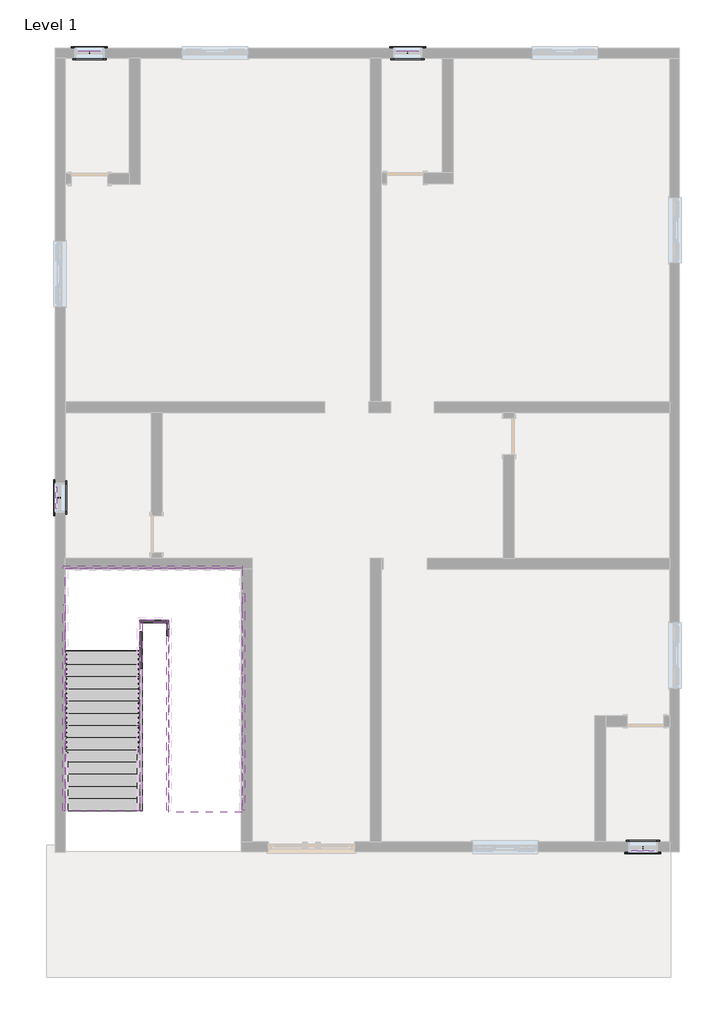
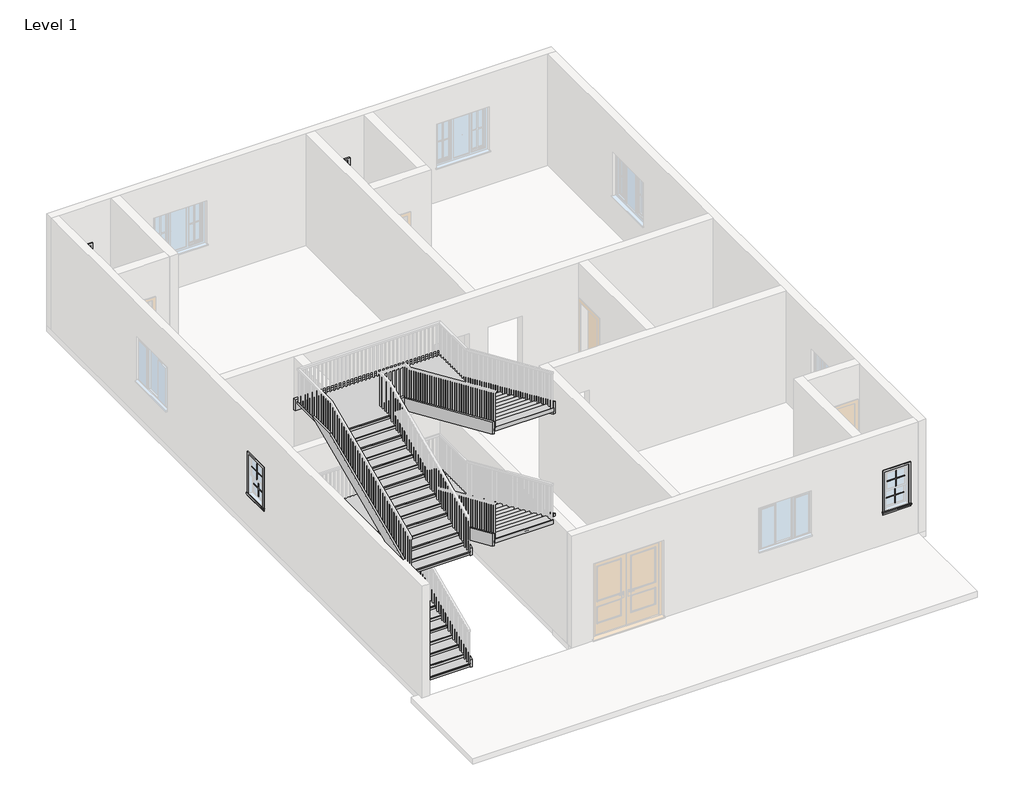
# One storey, part 6 of 6: 16 proxies, 12 members, 2 stair flights.
"""IFC4 building model written with IfcOpenShell, lengths in millimetres."""

from ifc_helpers import new_model, si_unit, frame, origin, place, context, project, spatial, polyline, outline, extrude, transform, mapped, element, save
from components import muntin_pattern_2x2_muntin_pattern_2x2_eba6c5fb, trim_window_exterior_flat_with_sill_278e6a94, trim_window_interior_flat_picture_frame_e9fd5f45, stair_flight_b71c2a3e, stair_flight_f7f46773

model = new_model("IFC4")

# Units and contexts
model_context = context("Model", 3, world=origin())
ifc_project = project(units=[si_unit("LENGTHUNIT", "METRE", prefix="MILLI")], contexts=[model_context])

# Site, building, storey
site = spatial("IfcSite", under=ifc_project)
building = spatial("IfcBuilding", under=site)
storey = spatial("IfcBuildingStorey", under=building, Name="Level 1", Elevation=0.0)

# Proxies
placement = place(None, origin())
muntin_pattern_2x2_muntin_pattern_2x2_shape = muntin_pattern_2x2_muntin_pattern_2x2_eba6c5fb(model_context)
element("IfcBuildingElementProxy", 1, Name="Muntin Pattern_2x2 : Muntin Pattern_2x2", ObjectType="Muntin Pattern_2x2 : Muntin Pattern_2x2", at=placement, inside=storey, context=model_context, shape_type="MappedRepresentation", body=[
    mapped(muntin_pattern_2x2_muntin_pattern_2x2_shape, transform((-7722.7165084, -455.2217109, 1470.025), x_axis=(0.0, 1.0, 0.0), y_axis=(-1.0, 0.0, 0.0), z_axis=(0.0, 0.0, 1.0))),
])
element("IfcBuildingElementProxy", 2, Name="Muntin Pattern_2x2 : Muntin Pattern_2x2", ObjectType="Muntin Pattern_2x2 : Muntin Pattern_2x2", at=placement, inside=storey, context=model_context, shape_type="MappedRepresentation", body=[
    mapped(muntin_pattern_2x2_muntin_pattern_2x2_shape, transform((-7678.2665084, -455.2217109, 990.6), x_axis=(0.0, 1.0, 0.0), y_axis=(-1.0, 0.0, 0.0), z_axis=(0.0, 0.0, 1.0))),
])
element("IfcBuildingElementProxy", 3, Name="Muntin Pattern_2x2 : Muntin Pattern_2x2", ObjectType="Muntin Pattern_2x2 : Muntin Pattern_2x2", at=placement, inside=storey, context=model_context, shape_type="MappedRepresentation", body=[
    mapped(muntin_pattern_2x2_muntin_pattern_2x2_shape, transform((-7046.4415084, 8872.5685985, 1470.025), x_axis=(1.0, 0.0, 0.0), y_axis=(0.0, 1.0, 0.0), z_axis=(0.0, 0.0, 1.0))),
])
element("IfcBuildingElementProxy", 4, Name="Muntin Pattern_2x2 : Muntin Pattern_2x2", ObjectType="Muntin Pattern_2x2 : Muntin Pattern_2x2", at=placement, inside=storey, context=model_context, shape_type="MappedRepresentation", body=[
    mapped(muntin_pattern_2x2_muntin_pattern_2x2_shape, transform((-7046.4415084, 8828.1185985, 990.6), x_axis=(1.0, 0.0, 0.0), y_axis=(0.0, 1.0, 0.0), z_axis=(0.0, 0.0, 1.0))),
])
element("IfcBuildingElementProxy", 5, Name="Muntin Pattern_2x2 : Muntin Pattern_2x2", ObjectType="Muntin Pattern_2x2 : Muntin Pattern_2x2", at=placement, inside=storey, context=model_context, shape_type="MappedRepresentation", body=[
    mapped(muntin_pattern_2x2_muntin_pattern_2x2_shape, transform((-417.0415084, 8872.5685985, 1470.025), x_axis=(1.0, 0.0, 0.0), y_axis=(0.0, 1.0, 0.0), z_axis=(0.0, 0.0, 1.0))),
])
element("IfcBuildingElementProxy", 6, Name="Muntin Pattern_2x2 : Muntin Pattern_2x2", ObjectType="Muntin Pattern_2x2 : Muntin Pattern_2x2", at=placement, inside=storey, context=model_context, shape_type="MappedRepresentation", body=[
    mapped(muntin_pattern_2x2_muntin_pattern_2x2_shape, transform((-417.0415084, 8828.1185985, 990.6), x_axis=(1.0, 0.0, 0.0), y_axis=(0.0, 1.0, 0.0), z_axis=(0.0, 0.0, 1.0))),
])
element("IfcBuildingElementProxy", 7, Name="Muntin Pattern_2x2 : Muntin Pattern_2x2", ObjectType="Muntin Pattern_2x2 : Muntin Pattern_2x2", at=placement, inside=storey, context=model_context, shape_type="MappedRepresentation", body=[
    mapped(muntin_pattern_2x2_muntin_pattern_2x2_shape, transform((4485.1584916, -7796.1814015, 1470.025), x_axis=(-1.0, 0.0, 0.0), y_axis=(0.0, -1.0, 0.0), z_axis=(0.0, 0.0, 1.0))),
])
element("IfcBuildingElementProxy", 8, Name="Muntin Pattern_2x2 : Muntin Pattern_2x2", ObjectType="Muntin Pattern_2x2 : Muntin Pattern_2x2", at=placement, inside=storey, context=model_context, shape_type="MappedRepresentation", body=[
    mapped(muntin_pattern_2x2_muntin_pattern_2x2_shape, transform((4485.1584916, -7751.7314015, 990.6), x_axis=(-1.0, 0.0, 0.0), y_axis=(0.0, -1.0, 0.0), z_axis=(0.0, 0.0, 1.0))),
])
trim_window_exterior_flat_with_sill_shape = trim_window_exterior_flat_with_sill_278e6a94(model_context)
element("IfcBuildingElementProxy", 9, Name="Trim-Window-Exterior-Flat : with Sill", ObjectType="Trim-Window-Exterior-Flat : with Sill", at=placement, inside=storey, context=model_context, shape_type="MappedRepresentation", body=[
    mapped(trim_window_exterior_flat_with_sill_shape, transform((-7757.6415084, -455.2217109, 1981.2), x_axis=(0.0, -1.0, 0.0), y_axis=(0.0, 0.0, 1.0), z_axis=(-1.0, 0.0, 0.0))),
])
element("IfcBuildingElementProxy", 10, Name="Trim-Window-Exterior-Flat : with Sill", ObjectType="Trim-Window-Exterior-Flat : with Sill", at=placement, inside=storey, context=model_context, shape_type="MappedRepresentation", body=[
    mapped(trim_window_exterior_flat_with_sill_shape, transform((-7046.4415084, 8907.4935985, 1981.2), x_axis=(-1.0, 0.0, 0.0), y_axis=(0.0, 0.0, 1.0), z_axis=(0.0, 1.0, 0.0))),
])
element("IfcBuildingElementProxy", 11, Name="Trim-Window-Exterior-Flat : with Sill", ObjectType="Trim-Window-Exterior-Flat : with Sill", at=placement, inside=storey, context=model_context, shape_type="MappedRepresentation", body=[
    mapped(trim_window_exterior_flat_with_sill_shape, transform((-417.0415084, 8907.4935985, 1981.2), x_axis=(-1.0, 0.0, 0.0), y_axis=(0.0, 0.0, 1.0), z_axis=(0.0, 1.0, 0.0))),
])
element("IfcBuildingElementProxy", 12, Name="Trim-Window-Exterior-Flat : with Sill", ObjectType="Trim-Window-Exterior-Flat : with Sill", at=placement, inside=storey, context=model_context, shape_type="MappedRepresentation", body=[
    mapped(trim_window_exterior_flat_with_sill_shape, transform((4485.1584916, -7831.1064015, 1981.2), x_axis=(1.0, 0.0, 0.0), y_axis=(0.0, 0.0, 1.0), z_axis=(0.0, -1.0, 0.0))),
])
trim_window_interior_flat_picture_frame_shape = trim_window_interior_flat_picture_frame_e9fd5f45(model_context)
element("IfcBuildingElementProxy", 13, Name="Trim-Window-Interior-Flat : Picture Frame", ObjectType="Trim-Window-Interior-Flat : Picture Frame", at=placement, inside=storey, context=model_context, shape_type="MappedRepresentation", body=[
    mapped(trim_window_interior_flat_picture_frame_shape, transform((-7554.4415084, -455.2217109, 1981.2), x_axis=(0.0, 1.0, 0.0), y_axis=(0.0, 0.0, 1.0), z_axis=(1.0, 0.0, 0.0))),
])
element("IfcBuildingElementProxy", 14, Name="Trim-Window-Interior-Flat : Picture Frame", ObjectType="Trim-Window-Interior-Flat : Picture Frame", at=placement, inside=storey, context=model_context, shape_type="MappedRepresentation", body=[
    mapped(trim_window_interior_flat_picture_frame_shape, transform((-7046.4415084, 8704.2935985, 1981.2), x_axis=(1.0, 0.0, 0.0), y_axis=(0.0, 0.0, 1.0), z_axis=(0.0, -1.0, 0.0))),
])
element("IfcBuildingElementProxy", 15, Name="Trim-Window-Interior-Flat : Picture Frame", ObjectType="Trim-Window-Interior-Flat : Picture Frame", at=placement, inside=storey, context=model_context, shape_type="MappedRepresentation", body=[
    mapped(trim_window_interior_flat_picture_frame_shape, transform((-417.0415084, 8704.2935985, 1981.2), x_axis=(1.0, 0.0, 0.0), y_axis=(0.0, 0.0, 1.0), z_axis=(0.0, -1.0, 0.0))),
])
element("IfcBuildingElementProxy", 16, Name="Trim-Window-Interior-Flat : Picture Frame", ObjectType="Trim-Window-Interior-Flat : Picture Frame", at=placement, inside=storey, context=model_context, shape_type="MappedRepresentation", body=[
    mapped(trim_window_interior_flat_picture_frame_shape, transform((4485.1584916, -7627.9064015, 1981.2), x_axis=(-1.0, 0.0, 0.0), y_axis=(0.0, 0.0, 1.0), z_axis=(0.0, 1.0, 0.0))),
])

# Members
element("IfcMember", 17, ObjectType="Stringer - 2\" Width", at=placement, inside=storey, context=model_context, shape_type="SweptSolid", body=[
    extrude(outline(polyline([(-6973.0610642, -304.8), (-6973.0610642, -105.9449185), (-3441.822613, 1447.8), (-2685.0041973, 1447.8), (-6668.1860155, -304.8), (-6973.0610642, -304.8)])), frame((-7605.2415084, 0.0, 0.0), z_axis=(1.0, 0.0, 0.0), x_axis=(0.0, 1.0, 0.0)), (0.0, 0.0, 1.0), 50.8),
])
element("IfcMember", 18, ObjectType="Stringer - 2\" Width", at=placement, inside=storey, context=model_context, shape_type="SweptSolid", body=[
    extrude(outline(polyline([(-7605.2415084, -1928.4217109), (-7605.2415084, -1877.6217109), (-3866.3290366, -1877.6217109), (-3866.3290366, -1928.4217109), (-7605.2415084, -1928.4217109)])), frame((0.0, 0.0, 1143.0), z_axis=(0.0, 0.0, 1.0), x_axis=(1.0, 0.0, 0.0)), (0.0, 0.0, 1.0), 304.8),
])
element("IfcMember", 19, ObjectType="Stringer - 2\" Width", at=placement, inside=storey, context=model_context, shape_type="SweptSolid", body=[
    extrude(outline(polyline([(-3202.3906584, 1143.0), (-6973.0610642, 2802.0949786), (-6973.0610642, 3135.0950815), (-2445.5722427, 1143.0), (-3202.3906584, 1143.0)])), frame((-3866.3290366, 0.0, 0.0), z_axis=(1.0, 0.0, 0.0), x_axis=(0.0, 1.0, 0.0)), (0.0, 0.0, 1.0), 50.8),
])
element("IfcMember", 20, ObjectType="Stringer - 2\" Width", at=placement, inside=storey, context=model_context, shape_type="SweptSolid", body=[
    extrude(outline(polyline([(-6973.0610642, -304.8), (-6973.0610642, -105.9449185), (-3441.822613, 1447.8), (-3061.4610642, 1447.8), (-3061.4610642, 1282.1589786), (-6668.1860155, -304.8), (-6973.0610642, -304.8)])), frame((-5999.9290366, 0.0, 0.0), z_axis=(1.0, 0.0, 0.0), x_axis=(0.0, 1.0, 0.0)), (0.0, 0.0, 1.0), 50.8),
])
element("IfcMember", 21, ObjectType="Stringer - 2\" Width", at=placement, inside=storey, context=model_context, shape_type="SweptSolid", body=[
    extrude(outline(polyline([(-5999.9290366, -3061.4610642), (-5999.9290366, -3010.6610642), (-5441.1290366, -3010.6610642), (-5441.1290366, -3061.4610642), (-5999.9290366, -3061.4610642)])), frame((0.0, 0.0, 1143.0), z_axis=(0.0, 0.0, 1.0), x_axis=(1.0, 0.0, 0.0)), (0.0, 0.0, 1.0), 304.8),
])
element("IfcMember", 22, ObjectType="Stringer - 2\" Width", at=placement, inside=storey, context=model_context, shape_type="SweptSolid", body=[
    extrude(outline(polyline([(-3010.6610642, 1391.6390815), (-3010.6610642, 1143.0), (-3202.3906584, 1143.0), (-6973.0610642, 2802.0949786), (-6973.0610642, 3135.0950815), (-3010.6610642, 1391.6390815)])), frame((-5441.1290366, 0.0, 0.0), z_axis=(1.0, 0.0, 0.0), x_axis=(0.0, 1.0, 0.0)), (0.0, 0.0, 1.0), 50.8),
])
element("IfcMember", 23, ObjectType="Stringer - 2\" Width", at=placement, inside=storey, context=model_context, shape_type="SweptSolid", body=[
    extrude(outline(polyline([(-6973.0610642, 2743.2), (-6973.0610642, 2942.0550815), (-3441.822613, 4495.8), (-2685.0041973, 4495.8), (-6668.1860155, 2743.2), (-6973.0610642, 2743.2)])), frame((-7605.2415084, 0.0, 0.0), z_axis=(1.0, 0.0, 0.0), x_axis=(0.0, 1.0, 0.0)), (0.0, 0.0, 1.0), 50.8),
])
element("IfcMember", 24, ObjectType="Stringer - 2\" Width", at=placement, inside=storey, context=model_context, shape_type="SweptSolid", body=[
    extrude(outline(polyline([(-7605.2415084, -1928.4217109), (-7605.2415084, -1877.6217109), (-3866.3290366, -1877.6217109), (-3866.3290366, -1928.4217109), (-7605.2415084, -1928.4217109)])), frame((0.0, 0.0, 4191.0), z_axis=(0.0, 0.0, 1.0), x_axis=(1.0, 0.0, 0.0)), (0.0, 0.0, 1.0), 304.8),
])
element("IfcMember", 25, ObjectType="Stringer - 2\" Width", at=placement, inside=storey, context=model_context, shape_type="SweptSolid", body=[
    extrude(outline(polyline([(-3202.3906584, 4191.0), (-6973.0610642, 5850.0949786), (-6973.0610642, 6183.0950815), (-2445.5722427, 4191.0), (-3202.3906584, 4191.0)])), frame((-3866.3290366, 0.0, 0.0), z_axis=(1.0, 0.0, 0.0), x_axis=(0.0, 1.0, 0.0)), (0.0, 0.0, 1.0), 50.8),
])
element("IfcMember", 26, ObjectType="Stringer - 2\" Width", at=placement, inside=storey, context=model_context, shape_type="SweptSolid", body=[
    extrude(outline(polyline([(-6973.0610642, 2743.2), (-6973.0610642, 2942.0550815), (-3441.822613, 4495.8), (-3061.4610642, 4495.8), (-3061.4610642, 4330.1589786), (-6668.1860155, 2743.2), (-6973.0610642, 2743.2)])), frame((-5999.9290366, 0.0, 0.0), z_axis=(1.0, 0.0, 0.0), x_axis=(0.0, 1.0, 0.0)), (0.0, 0.0, 1.0), 50.8),
])
element("IfcMember", 27, ObjectType="Stringer - 2\" Width", at=placement, inside=storey, context=model_context, shape_type="SweptSolid", body=[
    extrude(outline(polyline([(-5999.9290366, -3061.4610642), (-5999.9290366, -3010.6610642), (-5441.1290366, -3010.6610642), (-5441.1290366, -3061.4610642), (-5999.9290366, -3061.4610642)])), frame((0.0, 0.0, 4191.0), z_axis=(0.0, 0.0, 1.0), x_axis=(1.0, 0.0, 0.0)), (0.0, 0.0, 1.0), 304.8),
])
element("IfcMember", 28, ObjectType="Stringer - 2\" Width", at=placement, inside=storey, context=model_context, shape_type="SweptSolid", body=[
    extrude(outline(polyline([(-3010.6610642, 4439.6390815), (-3010.6610642, 4191.0), (-3202.3906584, 4191.0), (-6973.0610642, 5850.0949786), (-6973.0610642, 6183.0950815), (-3010.6610642, 4439.6390815)])), frame((-5441.1290366, 0.0, 0.0), z_axis=(1.0, 0.0, 0.0), x_axis=(0.0, 1.0, 0.0)), (0.0, 0.0, 1.0), 50.8),
])

# Stair flights
stair_flight_shape = stair_flight_b71c2a3e(model_context)
element("IfcStairFlight", 29, ObjectType="2\" Tread 1\" Nosing 1/4\" Riser", at=placement, inside=storey, context=model_context, shape_type="MappedRepresentation", body=[
    mapped(stair_flight_shape, transform((0.0, 0.0, 0.0), x_axis=(1.0, 0.0, 0.0), y_axis=(0.0, 1.0, 0.0), z_axis=(0.0, 0.0, 1.0))),
])
stair_flight_2_shape = stair_flight_f7f46773(model_context)
element("IfcStairFlight", 30, ObjectType="2\" Tread 1\" Nosing 1/4\" Riser", at=placement, inside=storey, context=model_context, shape_type="MappedRepresentation", body=[
    mapped(stair_flight_2_shape, transform((0.0, 0.0, 0.0), x_axis=(1.0, 0.0, 0.0), y_axis=(0.0, 1.0, 0.0), z_axis=(0.0, 0.0, 1.0))),
])

save(model, "model.ifc")

# Revit data of these elements
# Type "Muntin Pattern_2x2 : Muntin Pattern_2x2"
#   Width [instance default] = 4' - 0"
#   Thickness = 0' - 0 1/2"
#   Height [instance default] = 4' - 0"
#   Distance = 0' - 0 3/4"
#   Interior Material [instance default] = none
#   Exterior Material [instance default] = none
#   Default Elevation = 0
# Type "Trim-Window-Exterior-Flat : with Sill"
#   Trim Width = 0' - 2 1/4"
#   Trim Thickness_Picture Frame = 0' - 1 1/4"
#   Trim Thickness_with Sill = 0' - 0 3/4"
#   Sill Thickness = 0' - 1 1/4"
#   Opening Width [instance default] = 2' - 0"
#   Opening Height [instance default] = 3' - 0"
#   Default Elevation = 4' - 0"
#   Sill = yes
#   Picture Frame = no
#   Trim Material [instance default] = none
# Type "Trim-Window-Interior-Flat : Picture Frame"
#   Trim Thickness_Picture Frame = 0' - 1 1/4"
#   Trim Width = 0' - 2 1/4"
#   Trim Thickness_with Sill = 0' - 0 3/4"
#   Sill Thickness = 0' - 1 1/4"
#   Opening Width [instance default] = 2' - 0"
#   Opening Height [instance default] = 3' - 0"
#   Default Elevation = 4' - 0"
#   Sill = no
#   Picture Frame = yes
#   Trim Material [instance default] = none
# Elements 1, 2, 3, 4, 5, 6, 7, 8 (IfcBuildingElementProxy, "Muntin Pattern_2x2 : Muntin Pattern_2x2")
#   Width = 1' - 6"
#   Height = 1' - 5 1/8"
#   Interior Material = Wood - Stained
#   Exterior Material = Clad - White
#   Phase Created = New Construction
#   Materials on its faces: "Clad - White", "Wood - Stained"
# Elements 9, 10, 11, 12 (IfcBuildingElementProxy, "Trim-Window-Exterior-Flat : with Sill")
#   Opening Width = 2' - 0"
#   Opening Height = 3' - 6"
#   Trim Material = Clad - White
#   Phase Created = New Construction
#   Materials on its faces: "Clad - White"
# Elements 13, 14, 15, 16 (IfcBuildingElementProxy, "Trim-Window-Interior-Flat : Picture Frame")
#   Opening Width = 2' - 0"
#   Opening Height = 3' - 6"
#   Trim Material = Wood - Stained
#   Phase Created = New Construction
#   Materials on its faces: "Wood - Stained"
# Elements 17, 18, 19, 20, 21, 22, 23, 24, 25, 26, 27, 28 (IfcMember, "Stringer - 2\" Width")
#   Phase Created = New Construction
# Elements 29, 30 (IfcStairFlight, "2\" Tread 1\" Nosing 1/4\" Riser")
#   Phase Created = New Construction
# Materials
#   "Clad - White": class "Wood", colour RGB 242 242 238, transparency 0, Cost = 0
#   "Wood - Stained": class "Wood", colour RGB 224 178 126, transparency 0, Cost = 0
